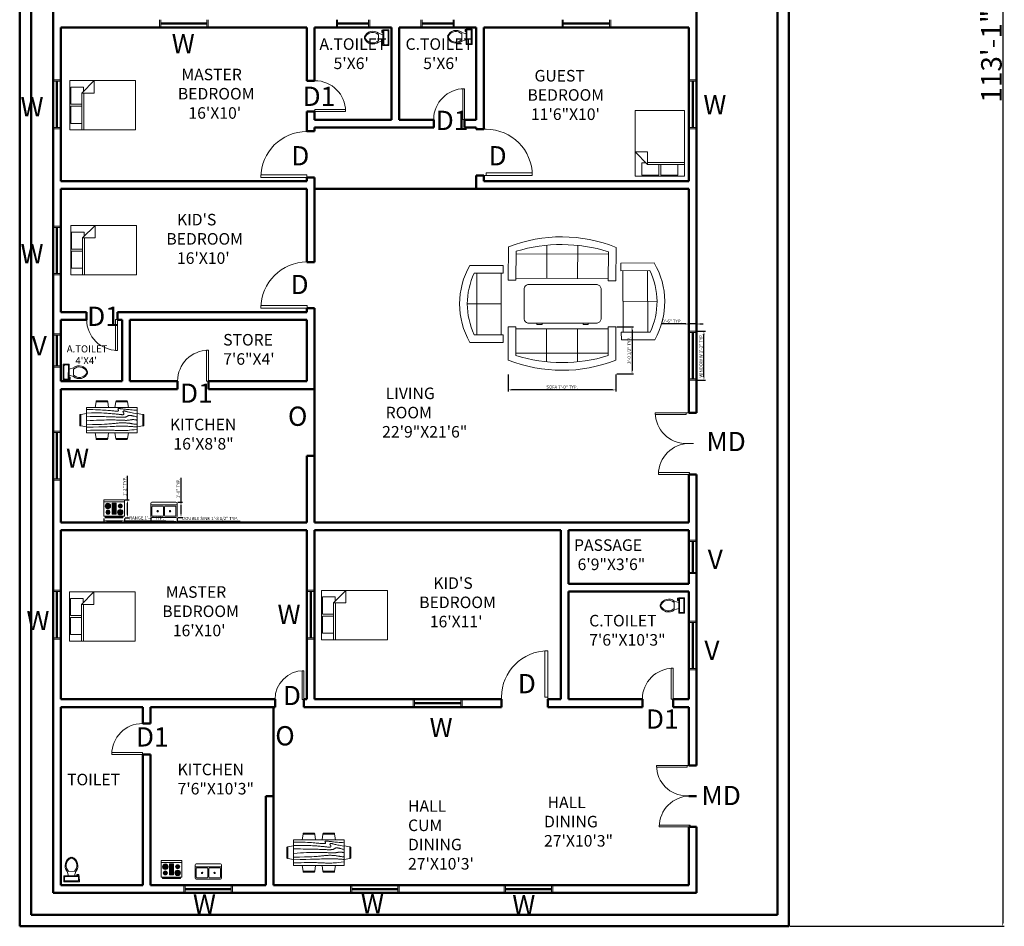
# Model space of a CAD drawing. Units: inches. Extents: x -7040 to -4088, y 6092 to 7645.
# Tile 8 of 11: x -5800 to -5032, y 6157 to 6864. Entities that reach past the tile are written whole.
import ezdxf

# ---------------------------------------------------------------- set-up
doc = ezdxf.new("R2010")
doc.units = ezdxf.units.IN
for name, color, linetype, lineweight in [('A-ANNO-DIMS', 2, 'Continuous', 18), ('A-ANNO-TEXT', 7, 'Continuous', 25), ('A-AREA-IDEN', 3, 'Continuous', 25), ('A-DOOR', 3, 'Continuous', 18), ('A-FLOR-FIXT', 9, 'Continuous', 13), ('A-FURN', 8, 'Continuous', 13), ('A-GLAZ', 4, 'Continuous', 18), ('A-WALL', 7, 'Continuous', 50)]:
    doc.layers.add(name, color=color, linetype=linetype, lineweight=lineweight)
doc.styles.get("Standard").update_dxf_attribs({"font": 'arial.ttf'})
doc.dimstyles.new('ISO-25', dxfattribs={"dimtxt": 2.5, "dimasz": 2.5, "dimexe": 1.25, "dimexo": 0.625, "dimtad": 1, "dimdec": 0, "dimlunit": 3, "dimtxsty": 'Standard', "dimcen": 2.5, "dimadec": 0, "dimazin": 0, "dimtfac": 1, "dimtdec": 0, "dimtmove": 0, "dimatfit": 3, "dimfxl": 1, "dimarcsym": 0})

# ---------------------------------------------------------------- blocks, each defined once
blk = doc.blocks.new('*U8')
for p, q in [((0, 0), (0, -100)), ((750, 0), (750, -100))]:
    blk.add_line(p, q)
blk.add_lwpolyline([(0, 0), (0, 750), (43.75, 750), (43.75, 0)], close=True)
blk.add_arc((0, 0), 750, 0, 90)
blk = doc.blocks.new('Bed - Queen')
for p, q in [((0, -80.00003), (0, 0)), ((0, 0), (59.99999, 0)), ((59.99999, 0), (59.99999, -80.00003)), ((7.99999, -1.2), (28.79998, -1.2)), ((7.99999, -14.4), (7.99999, -1.2)), ((28.79998, -1.2), (28.79998, -14.4)), ((31.19999, -1.2), (51.99999, -1.2)), ((31.19999, -14.4), (31.19999, -1.2)), ((51.99999, -1.2), (51.99999, -16.4)), ((0, -14.4), (44.8, -14.4)), ((44.8, -16.8), (0, -16.8)), ((59.99999, -29.6), (44.8, -14.4)), ((44.8, -14.4), (44.8, -29.6)), ((51.99999, -16.4), (46.79936, -16.4)), ((44.8, -29.6), (59.99999, -29.6)), ((59.99999, -80.00003), (0, -80.00003))]:
    blk.add_line(p, q)
blk = doc.blocks.new('Range-Oven - 30 in top')
for p, q in [((0, -3), (30, -3)), ((12, -6), (18, -6)), ((13, -20), (13, -6)), ((14, -6), (14, -20)), ((15, -20), (15, -6)), ((16, -6), (16, -20)), ((17, -20), (17, -6)), ((6, -24), (6, -25)), ((8, -25), (8, -24)), ((18, -20), (12, -20)), ((22, -25), (22, -24)), ((24, -24), (24, -25))]:
    blk.add_line(p, q)
for points in [[(0, -24), (0, 0), (30, 0), (30, -24)], [(12, -21), (12, -5), (18, -5), (18, -21)], [(2, -26), (2, -25), (28, -25), (28, -26)]]:
    blk.add_lwpolyline(points, close=True)
for centre, radius in [((6, -9), 4), ((6, -9), 3), ((6, -9), 2), ((6, -9), 1), ((24, -18), 4), ((24, -9), 3), ((24, -9), 2), ((24, -9), 1), ((6, -18), 3), ((6, -18), 2), ((6, -18), 1), ((24, -18), 3), ((24, -18), 2), ((24, -18), 1)]:
    blk.add_circle(centre, radius)
blk = doc.blocks.new('Sink-double - 36 in top')
for p, q in [((-18, -4), (18, -4)), ((-0.75, -18.5), (-0.75, -6.5)), ((0.75, -6.5), (0.75, -18.5))]:
    blk.add_line(p, q)
for points in [[(-16.5, 0), (16.5, 0)], [(-18, -19.5), (-18, -1.5)], [(-16.5, -18.5), (-16.5, -6.5)], [(-15.5, -5.5), (-1.75, -5.5)], [(1.75, -5.5), (15.5, -5.5)], [(16.5, -6.5), (16.5, -18.5)], [(18, -1.5), (18, -19.5)], [(16.5, -21), (-16.5, -21)], [(-1.75, -19.5), (-15.5, -19.5)], [(15.5, -19.5), (1.75, -19.5)]]:
    blk.add_lwpolyline(points)
for centre, radius in [((-8.5, -12.5), 1), ((-8.5, -12.5), 0.5), ((8.5, -12.5), 1), ((8.5, -12.5), 0.5)]:
    blk.add_circle(centre, radius)
for centre, radius, start, end in [((-16.5, -1.5), 1.5, 90, 180), ((16.5, -1.5), 1.5, 0, 90), ((-15.5, -6.5), 1, 90, 180), ((-1.75, -6.5), 1, 0, 90), ((1.75, -6.5), 1, 90, 180), ((15.5, -6.5), 1, 0, 90), ((-16.5, -19.5), 1.5, 180, 270), ((-15.5, -18.5), 1, 180, 270), ((-1.75, -18.5), 1, 270, 0), ((1.75, -18.5), 1, 180, 270), ((15.5, -18.5), 1, 270, 0), ((16.5, -19.5), 1.5, 270, 0)]:
    blk.add_arc(centre, radius, start, end)
blk = doc.blocks.new('Toilet - top')
for p, q in [((-10, -8.5), (-8, -8.5)), ((-10, -9.5), (-10, -8.5)), ((-7, -9.5), (-10, -9.5)), ((-8, -8.5), (-8, -8)), ((-7, -8), (-7, -9.5)), ((-4, -8), (-6, -14)), ((4, -8), (6, -14)), ((9.5, -6), (9.5, -2)), ((4, -14), (-4, -14))]:
    blk.add_line(p, q)
blk.add_lwpolyline([(10.5, -8), (10.5, 0), (-10.5, 0), (-10.5, -8)], close=True)
for points in [[(-9.5, -2), (-9.5, -6)], [(8.5, -1), (-8.5, -1)], [(-8.5, -7), (8.5, -7)]]:
    blk.add_lwpolyline(points)
for centre, radius, start, end in [((-8.6, -1.9), 0.884, 81.8699, 188.1301), ((-8.6, -6.1), 0.884, 171.8699, 278.1301), ((8.6, -1.9), 0.884, 351.8699, 98.1301), ((8.6, -6.1), 0.884, 261.8699, 8.1301), ((3.5, -21.6), 12.2, 141.4691, 247.9714), ((4.2, -21.8), 11.3, 136.3677, 238.9468), ((-3.5, -21.6), 12.2, 292.0284, 38.5307), ((-4.2, -21.8), 11.3, 301.053, 43.6321), ((0, -27.9), 4, 245.7318, 294.2682), ((0, -29), 4, 254.8605, 285.1395)]:
    blk.add_arc(centre, radius, start, end)
blk = doc.blocks.new('Dining Set - 36 x 72 in.')
for p, q in [((36, 18), (-36, 18)), ((-36, 18), (-36, -18)), ((-22.2343, 26.00059), (-23.4847, 17.99762)), ((-22.2304, 26), (-5.7608, 26)), ((-22, 27.5), (-22.1562, 26.50042)), ((-5.8416, 26.5), (-22.1534, 26.5)), ((-22, 27.5), (-6, 27.5)), ((-5.8437, 26.49966), (-6, 27.5)), ((-4.5152, 17.99762), (-5.7655, 25.99926)), ((5.7657, 26.00059), (4.5153, 17.99762)), ((5.7696, 26), (22.2392, 26)), ((6, 27.5), (5.8438, 26.50042)), ((22.1584, 26.5), (5.8466, 26.5)), ((6, 27.5), (22, 27.5)), ((22.1563, 26.49966), (22, 27.5)), ((23.4848, 17.99762), (22.2345, 25.99926)), ((36, -18), (36, 18)), ((-45.5, 8), (-44.5004, 8.15617)), ((-45.5, 8), (-45.5, -8)), ((-44.5, -8.15843), (-44.5, 8.15338)), ((-44.0006, 8.23428), (-35.9976, 9.48474)), ((-44, 8.23041), (-44, -8.23915)), ((44.0006, 8.23428), (35.9976, 9.48474)), ((44, 8.23041), (44, -8.23915)), ((44.5, -8.15843), (44.5, 8.15338)), ((45.5, 8), (44.5005, 8.15617)), ((45.5, 8), (45.5, -8)), ((-44.4997, -8.15631), (-45.5, -8)), ((-35.9976, -9.48476), (-43.9993, -8.2345)), ((35.9976, -9.48476), (43.9993, -8.2345)), ((44.4997, -8.15631), (45.5, -8)), ((-36, -18), (36, -18)), ((-22.2343, -26.0006), (-23.4847, -17.99762)), ((-22.2304, -26), (-5.7608, -26)), ((-22, -27.5), (-22.1562, -26.50044)), ((-5.8416, -26.5), (-22.1534, -26.5)), ((-22, -27.5), (-6, -27.5)), ((-5.8437, -26.49967), (-6, -27.5)), ((-4.5152, -17.99762), (-5.7655, -25.99928)), ((5.7657, -26.0006), (4.5153, -17.99762)), ((5.7696, -26), (22.2392, -26)), ((6, -27.5), (5.8438, -26.50044)), ((22.1584, -26.5), (5.8466, -26.5)), ((6, -27.5), (22, -27.5)), ((22.1563, -26.49967), (22, -27.5)), ((23.4848, -17.99762), (22.2345, -25.99928))]:
    blk.add_line(p, q)
for points in [[(-36, 15), (-31.1772, 14.97754), (-26.8079, 14.91406), (-22.8538, 14.81543), (-19.276, 14.6875), (-16.0362, 14.53613), (-13.0957, 14.36718), (-10.4159, 14.18652), (-7.9583, 14), (-5.6904, 13.81315), (-3.6035, 13.63021), (-1.6954, 13.45508), (0.0365, 13.29166), (1.5945, 13.14388), (2.9811, 13.01562), (4.1988, 12.9108), (5.25, 12.83333), (6.1393, 12.78613), (6.8802, 12.76823), (7.4883, 12.77767), (7.9792, 12.8125), (8.3685, 12.87077), (8.6719, 12.95052), (8.9049, 13.0498), (9.0833, 13.16666), (9.2205, 13.29899), (9.3216, 13.44401), (9.3895, 13.59879), (9.4271, 13.76041), (9.4373, 13.92594), (9.4232, 14.09245), (9.3875, 14.257), (9.3333, 14.41666), (9.2638, 14.56917), (9.1836, 14.71484), (9.0975, 14.85465), (9.0104, 14.98958), (8.9272, 15.1206), (8.8529, 15.2487), (8.7922, 15.37483), (8.75, 15.5), (8.7305, 15.62467), (8.7344, 15.74739), (8.7617, 15.86621), (8.8125, 15.97916), (8.8867, 16.08431), (8.9844, 16.17968), (9.1055, 16.26334), (9.25, 16.33333), (9.4189, 16.38802), (9.6172, 16.42708), (9.8506, 16.45052), (10.125, 16.45833), (10.4463, 16.45052), (10.8203, 16.42708), (11.2529, 16.38802), (11.75, 16.33333), (12.3184, 16.26318), (12.9694, 16.17838), (13.7151, 16.07991), (14.5677, 15.96875), (15.5395, 15.84586), (16.6426, 15.71224), (17.8893, 15.56884), (19.2917, 15.41666), (20.859, 15.25667), (22.5879, 15.08984), (24.4721, 14.91715), (26.5052, 14.73958), (28.6809, 14.5581), (30.9929, 14.3737), (33.4347, 14.18733), (36, 14)], [(-36, 10), (-28.9766, 10.14274), (-23.1725, 10.20442), (-18.4241, 10.19775), (-14.5677, 10.13541), (-11.4399, 10.03011), (-8.877, 9.89453), (-6.7154, 9.74137), (-4.7917, 9.58333), (-2.9698, 9.43082), (-1.2246, 9.28515), (0.4415, 9.14534), (2.026, 9.01041), (3.5266, 8.87939), (4.9408, 8.7513), (6.266, 8.62516), (7.5, 8.5), (8.6411, 8.37549), (9.6914, 8.2539), (10.6538, 8.13818), (11.5312, 8.03125), (12.3267, 7.93603), (13.043, 7.85547), (13.6831, 7.79248), (14.25, 7.75), (14.7471, 7.7303), (15.1797, 7.73307), (15.5537, 7.75732), (15.875, 7.80208), (16.1494, 7.86637), (16.3828, 7.94922), (16.5811, 8.04964), (16.75, 8.16666), (16.8944, 8.29915), (17.0143, 8.44531), (17.1089, 8.60319), (17.1771, 8.77083), (17.218, 8.94629), (17.2305, 9.1276), (17.2137, 9.31282), (17.1667, 9.5), (17.0895, 9.6875), (16.987, 9.875), (16.8649, 10.0625), (16.7292, 10.25), (16.5856, 10.4375), (16.4401, 10.625), (16.2985, 10.8125), (16.1667, 11), (16.05, 11.18733), (15.9518, 11.3737), (15.8752, 11.5581), (15.8229, 11.73958), (15.798, 11.91715), (15.8034, 12.08984), (15.842, 12.25667), (15.9167, 12.41666), (16.0295, 12.56836), (16.1784, 12.70833), (16.3605, 12.83268), (16.5729, 12.9375), (16.8127, 13.01888), (17.0768, 13.07291), (17.3625, 13.0957), (17.6667, 13.08333), (17.9894, 13.03312), (18.3418, 12.94726), (18.7382, 12.82918), (19.1927, 12.68229), (19.7195, 12.51001), (20.3327, 12.31575), (21.0465, 12.10294), (21.875, 11.875), (22.8357, 11.63354), (23.959, 11.37304), (25.2786, 11.08618), (26.8282, 10.76562), (28.6414, 10.40405), (30.752, 9.99414), (33.1936, 9.52856), (36, 9)], [(-36, 5.5), (-30.7157, 5.3348), (-26.069, 5.20963), (-21.9946, 5.11767), (-18.4271, 5.05208), (-15.3009, 5.00602), (-12.5508, 4.97265), (-10.1112, 4.94515), (-7.9167, 4.91666), (-5.909, 4.88167), (-4.0586, 4.83984), (-2.3429, 4.79215), (-0.7396, 4.73958), (0.7739, 4.6831), (2.22, 4.6237), (3.6213, 4.56233), (5, 4.5), (6.373, 4.43782), (7.7344, 4.3776), (9.0723, 4.32129), (10.375, 4.27083), (11.6309, 4.22819), (12.8281, 4.19531), (13.9551, 4.17415), (15, 4.16666), (15.954, 4.17448), (16.819, 4.19791), (17.6001, 4.23698), (18.3021, 4.29166), (18.9299, 4.36198), (19.4883, 4.44791), (19.9823, 4.54948), (20.4167, 4.66666), (20.7969, 4.79899), (21.1302, 4.94401), (21.4245, 5.09879), (21.6875, 5.26041), (21.9271, 5.42594), (22.1511, 5.59245), (22.3672, 5.757), (22.5834, 5.91666), (22.8065, 6.06868), (23.0404, 6.21093), (23.2879, 6.34147), (23.5521, 6.45833), (23.8358, 6.55957), (24.142, 6.64323), (24.4735, 6.70735), (24.8334, 6.75), (25.2235, 6.76969), (25.642, 6.76692), (26.0858, 6.74267), (26.5521, 6.69791), (27.0379, 6.63362), (27.5404, 6.55078), (28.0565, 6.45036), (28.5834, 6.33333), (29.1242, 6.19987), (29.7071, 6.04687), (30.3661, 5.87044), (31.1354, 5.66666), (32.0493, 5.43164), (33.142, 5.16146), (34.4475, 4.85221), (36, 4.5)], [(-36, -1), (-30.7915, -0.6591), (-26.0195, -0.38216), (-21.6519, -0.16284), (-17.6563, 0.00521), (-14.0005, 0.12833), (-10.6523, 0.21289), (-7.5796, 0.26522), (-4.75, 0.29166), (-2.134, 0.29793), (0.2878, 0.28711), (2.5317, 0.26163), (4.6146, 0.22396), (6.5529, 0.17651), (8.3633, 0.12174), (10.0623, 0.06209), (11.6667, 0), (13.1899, -0.06201), (14.6341, -0.1211), (15.9982, -0.17432), (17.2813, -0.21875), (18.4823, -0.25147), (19.6003, -0.26953), (20.6343, -0.27002), (21.5834, -0.25), (22.4481, -0.20768), (23.2357, -0.14584), (23.9549, -0.06836), (24.6146, 0.02083), (25.2235, 0.11784), (25.7904, 0.21875), (26.3241, 0.31966), (26.8334, 0.41666), (27.3265, 0.50618), (27.8099, 0.58593), (28.2894, 0.65397), (28.7709, 0.70833), (29.2601, 0.74707), (29.763, 0.76823), (30.2855, 0.76985), (30.8334, 0.75), (31.4088, 0.70784), (31.9994, 0.64713), (32.589, 0.57275), (33.1615, 0.48958), (33.7008, 0.4025), (34.1908, 0.3164), (34.6153, 0.23616), (34.9584, 0.16666), (35.2099, 0.11165), (35.3848, 0.07031), (35.504, 0.04069), (35.5886, 0.02083), (35.6594, 0.00879), (35.7377, 0.0026), (35.8442, 0.00032), (36, 0)], [(-36, -6.5), (-27.1843, -6.31267), (-20.084, -6.1263), (-14.469, -5.9419), (-10.1094, -5.76042), (-6.7752, -5.58285), (-4.2363, -5.41016), (-2.2629, -5.24333), (-0.625, -5.08334), (0.8708, -4.93099), (2.2715, -4.78646), (3.5872, -4.64974), (4.8281, -4.52084), (6.0046, -4.39974), (7.127, -4.28646), (8.2053, -4.18099), (9.25, -4.08334), (10.2705, -3.99382), (11.2734, -3.91407), (12.2647, -3.84603), (13.25, -3.79167), (14.2354, -3.75293), (15.2266, -3.73177), (16.2295, -3.73015), (17.25, -3.75), (18.2912, -3.79248), (19.3451, -3.85547), (20.4009, -3.93604), (21.4479, -4.03125), (22.4754, -4.13819), (23.4727, -4.25391), (24.4289, -4.37549), (25.3334, -4.5), (26.1785, -4.62492), (26.9694, -4.74935), (27.7145, -4.87281), (28.4219, -4.99479), (29.1, -5.11483), (29.7572, -5.23242), (30.4016, -5.34709), (31.0417, -5.45834), (31.6837, -5.56437), (32.3262, -5.65821), (32.9658, -5.73153), (33.599, -5.77604), (34.2224, -5.78345), (34.8327, -5.74545), (35.4264, -5.65373), (36, -5.5)], [(-36, -10), (-26.4022, -9.81299), (-18.4675, -9.62891), (-11.9839, -9.45069), (-6.7396, -9.28125), (-2.5226, -9.12354), (0.8789, -8.98047), (3.6769, -8.85498), (6.0833, -8.75), (8.2767, -8.66765), (10.3021, -8.60677), (12.1712, -8.56543), (13.8958, -8.54167), (15.4876, -8.53353), (16.9583, -8.53907), (18.3197, -8.55632), (19.5834, -8.58334), (20.7616, -8.61841), (21.8685, -8.66081), (22.9188, -8.71004), (23.9271, -8.76563), (24.9081, -8.82707), (25.8763, -8.89388), (26.8465, -8.96558), (27.8334, -9.04167), (28.8474, -9.12118), (29.8828, -9.20117), (30.93, -9.27824), (31.9792, -9.34896), (33.0205, -9.40991), (34.0443, -9.45768), (35.0407, -9.48885), (36, -9.5)], [(-36, -14.5), (-30.0881, -14.33513), (-25.0332, -14.21224), (-20.7312, -14.12647), (-17.0781, -14.07292), (-13.97, -14.04671), (-11.3027, -14.04297), (-8.9724, -14.05681), (-6.875, -14.08334), (-4.9224, -14.11833), (-3.0905, -14.16016), (-1.3709, -14.20785), (0.2448, -14.26042), (1.7647, -14.3169), (3.1973, -14.3763), (4.5507, -14.43767), (5.8333, -14.5), (7.0554, -14.5621), (8.235, -14.62175), (9.3922, -14.67652), (10.5469, -14.72396), (11.7192, -14.76164), (12.929, -14.78711), (14.1965, -14.79794), (15.5417, -14.79167), (16.9933, -14.76424), (18.6152, -14.70508), (20.4804, -14.60197), (22.6615, -14.44271), (25.2312, -14.21509), (28.2624, -13.9069), (31.8277, -13.50594), (36, -13)]]:
    blk.add_lwpolyline(points)
blk = doc.blocks.new('Desk - 30 x 60 in.')
for p, q in [((-26.999995, 0), (26.999995, 0)), ((-29.999995, -27), (-29.999995, -3)), ((29.999995, -3), (29.999995, -27)), ((26.999995, -30), (-26.999995, -30)), ((-20.000005, -30), (-20.000005, -31)), ((-16.000005, -31), (-16.000005, -30)), ((15.999995, -31), (15.999995, -30)), ((19.999995, -30), (19.999995, -31)), ((-20.000005, -31), (-16.000005, -31)), ((19.999995, -31), (15.999995, -31))]:
    blk.add_line(p, q)
for centre, start, end in [((-26.499995, -3.5), 98.1301, 171.8699), ((26.499995, -3.5), 8.130102, 81.8699), ((-26.499995, -26.5), 188.1301, 261.8699), ((26.499995, -26.5), 278.1301, 351.8699)]:
    blk.add_arc(centre, 3.535534, start, end)
blk = doc.blocks.new('Sofa - Roundback 7 ft.')
for p, q in [((-12.00002, -32.4421), (-12.00003, -6.5971)), ((11.99997, -32.4421), (11.99998, -6.5971)), ((-36.000027, -34), (-36.000027, -11.4696)), ((-35.999844, -13.3819), (35.9998, -13.3819)), ((35.99998, -34), (35.99998, -11.4696)), ((-36.000027, -32.4421), (35.99998, -32.4421))]:
    blk.add_line(p, q)
for points in [[(-36.000027, -34), (-42.000027, -34), (-42.000027, -8)], [(41.99998, -8), (41.99998, -34), (35.99998, -34)]]:
    blk.add_lwpolyline(points)
for centre, radius, start, end in [((0, -114.25), 114.25, 68.43141, 111.5686), ((-0.00001, -127.1968), 121.1968, 72.72033, 107.2797)]:
    blk.add_arc(centre, radius, start, end)
blk = doc.blocks.new('Sofa - Roundback Loveseat 5 ft.')
for p, q in [((0, -32.44198), (0, -5.99998)), ((-24, -33.99998), (-24, -11.46958)), ((-23.9998, -13.38178), (23.99986, -13.38178)), ((24.00004, -33.99998), (24.00004, -11.46958)), ((-24, -32.44198), (24.00004, -32.44198))]:
    blk.add_line(p, q)
for points in [[(-24, -33.99998), (-30, -33.99998), (-30, -7.99998)], [(30.00004, -7.99998), (30.00004, -33.99998), (24.00004, -33.99998)]]:
    blk.add_lwpolyline(points)
for centre, radius, start, end in [((0, -60.24998), 60.24998, 60.13715, 119.8628), ((0, -61.38438), 55.38444, 64.32083, 115.6792)]:
    blk.add_arc(centre, radius, start, end)
blk = doc.blocks.new('*D102')
at = {"layer": 'A-ANNO-DIMS', "color": 0, "lineweight": -2, "transparency": 16777216}
for p, q in [((-5199.27, 7513.76), (-5031.95, 7513.76)), ((-5033.2, 7511.26), (-5033.2, 6159.26)), ((-5199.27, 6156.76), (-5031.95, 6156.76))]:
    blk.add_line(p, q, dxfattribs=at)
at = {"layer": 'A-ANNO-DIMS', "color": 0, "transparency": 16777216}
for points in [[(-5033.61, 7511.26), (-5032.78, 7511.26), (-5033.2, 7513.76)], [(-5033.61, 6159.26), (-5032.78, 6159.26), (-5033.2, 6156.76)]]:
    blk.add_solid(points, dxfattribs=at)
at = {"layer": 'Defpoints', "color": 0, "transparency": 16777216}
for p in [(-5199.9, 7513.76), (-5199.9, 6156.76), (-5033.2, 6156.76)]:
    blk.add_point(p, dxfattribs=at)
at = {"layer": 'A-ANNO-DIMS', "color": 0, "transparency": 16777216, "insert": (-5042, 6835.26), "char_height": 2.5, "attachment_point": 5, "rotation": 90}
blk.add_mtext('{\\H6.4x;113\'-1"}', dxfattribs=at)
blk = doc.blocks.new('WIN-36')
for p, q in [((0, 6), (0, 0)), ((1, 6), (1, 0)), ((1, 3.5), (37, 3.5)), ((1, 3), (37, 3)), ((1, 2.5), (37, 2.5)), ((37, 6), (37, 0)), ((38, 6), (38, 0))]:
    blk.add_line(p, q)
blk = doc.blocks.new('WIN-24')
for p, q in [((0, 6), (0, 0)), ((1, 6), (1, 0)), ((1, 3.5), (25, 3.5)), ((1, 3), (25, 3)), ((1, 2.5), (25, 2.5)), ((25, 6), (25, 0)), ((26, 6), (26, 0))]:
    blk.add_line(p, q)
blk = doc.blocks.new('*D114')
at = {"layer": 'A-ANNO-DIMS', "color": 0, "lineweight": -2, "transparency": 16777216}
for p, q in [((-5271.27, 6620.76), (-5264.95, 6620.76)), ((-5266.2, 6585.26), (-5266.2, 6618.26)), ((-5271.27, 6582.76), (-5264.95, 6582.76))]:
    blk.add_line(p, q, dxfattribs=at)
at = {"layer": 'A-ANNO-DIMS', "color": 0, "transparency": 16777216}
for points in [[(-5266.62, 6618.26), (-5265.78, 6618.26), (-5266.2, 6620.76)], [(-5266.62, 6585.26), (-5265.78, 6585.26), (-5266.2, 6582.76)]]:
    blk.add_solid(points, dxfattribs=at)
at = {"layer": 'Defpoints', "color": 0, "transparency": 16777216}
for p in [(-5271.9, 6620.76), (-5266.2, 6620.76), (-5271.9, 6582.76)]:
    blk.add_point(p, dxfattribs=at)
at = {"layer": 'A-ANNO-DIMS', "color": 0, "transparency": 16777216, "insert": (-5268.12, 6601.76), "char_height": 2.5, "attachment_point": 5, "rotation": 90}
blk.add_mtext('WINDOW W 3\'-2" TYP.', dxfattribs=at)
blk = doc.blocks.new('*D115')
at = {"layer": 'A-ANNO-DIMS', "color": 0, "lineweight": -2, "transparency": 16777216}
for p, q in [((-5277.9, 6621.38), (-5277.9, 6627.71)), ((-5271.9, 6621.38), (-5271.9, 6627.71)), ((-5280.4, 6626.46), (-5299.39, 6626.46)), ((-5271.9, 6626.46), (-5277.9, 6626.46)), ((-5269.4, 6626.46), (-5266.9, 6626.46))]:
    blk.add_line(p, q, dxfattribs=at)
at = {"layer": 'A-ANNO-DIMS', "color": 0, "transparency": 16777216}
for points in [[(-5280.4, 6626.88), (-5280.4, 6626.04), (-5277.9, 6626.46)], [(-5269.4, 6626.88), (-5269.4, 6626.04), (-5271.9, 6626.46)]]:
    blk.add_solid(points, dxfattribs=at)
at = {"layer": 'Defpoints', "color": 0, "transparency": 16777216}
for p in [(-5277.9, 6626.46), (-5277.9, 6620.76), (-5271.9, 6620.76)]:
    blk.add_point(p, dxfattribs=at)
at = {"layer": 'A-ANNO-DIMS', "color": 0, "transparency": 16777216, "insert": (-5291.14, 6628.36), "char_height": 2.5, "attachment_point": 5}
blk.add_mtext('0\'-6" TYP.', dxfattribs=at)
blk = doc.blocks.new('*D138')
at = {"layer": 'A-ANNO-DIMS', "color": 0, "lineweight": -2, "transparency": 16777216}
for p, q in [((-5418.91, 6587.05), (-5418.91, 6573.83)), ((-5334.91, 6587.04), (-5334.91, 6573.81)), ((-5337.41, 6575.06), (-5416.41, 6575.08))]:
    blk.add_line(p, q, dxfattribs=at)
at = {"layer": 'A-ANNO-DIMS', "color": 0, "transparency": 16777216}
for points in [[(-5416.41, 6575.49), (-5416.41, 6574.66), (-5418.91, 6575.08)], [(-5337.41, 6575.48), (-5337.41, 6574.64), (-5334.91, 6575.06)]]:
    blk.add_solid(points, dxfattribs=at)
at = {"layer": 'Defpoints', "color": 0, "transparency": 16777216}
for p in [(-5418.91, 6587.68), (-5334.91, 6587.66), (-5418.91, 6575.08)]:
    blk.add_point(p, dxfattribs=at)
at = {"layer": 'A-ANNO-DIMS', "color": 0, "transparency": 16777216, "insert": (-5376.91, 6576.99), "char_height": 2.5, "attachment_point": 5, "rotation": 359.98844}
blk.add_mtext('SOFA 7\'-0" TYP.', dxfattribs=at)
blk = doc.blocks.new('*D139')
at = {"layer": 'A-ANNO-DIMS', "color": 0, "lineweight": -2, "transparency": 16777216}
for p, q in [((-5334.28, 6624.33), (-5321.05, 6624.32)), ((-5322.3, 6621.82), (-5322.31, 6590.16)), ((-5334.28, 6587.66), (-5321.06, 6587.66))]:
    blk.add_line(p, q, dxfattribs=at)
at = {"layer": 'A-ANNO-DIMS', "color": 0, "transparency": 16777216}
for points in [[(-5322.72, 6621.82), (-5321.88, 6621.82), (-5322.3, 6624.32)], [(-5322.72, 6590.16), (-5321.89, 6590.16), (-5322.31, 6587.66)]]:
    blk.add_solid(points, dxfattribs=at)
at = {"layer": 'Defpoints', "color": 0, "transparency": 16777216}
for p in [(-5334.9, 6624.33), (-5334.91, 6587.66), (-5322.31, 6587.66)]:
    blk.add_point(p, dxfattribs=at)
at = {"layer": 'A-ANNO-DIMS', "color": 0, "transparency": 16777216, "insert": (-5324.22, 6605.99), "char_height": 2.5, "attachment_point": 5, "rotation": 89.98844}
blk.add_mtext('3\'-0 1/2" TYP.', dxfattribs=at)
blk = doc.blocks.new('*D150')
at = {"layer": 'A-ANNO-DIMS', "color": 0, "lineweight": -2, "transparency": 16777216}
for p, q in [((-5734.29, 6474.79), (-5734.29, 6471.76)), ((-5718.26, 6474.79), (-5718.26, 6471.76)), ((-5731.79, 6473.01), (-5720.76, 6473.01)), ((-5718.26, 6473.01), (-5686.01, 6473.01))]:
    blk.add_line(p, q, dxfattribs=at)
at = {"layer": 'A-ANNO-DIMS', "color": 0, "transparency": 16777216}
for points in [[(-5731.79, 6473.42), (-5731.79, 6472.59), (-5734.29, 6473.01)], [(-5720.76, 6473.42), (-5720.76, 6472.59), (-5718.26, 6473.01)]]:
    blk.add_solid(points, dxfattribs=at)
at = {"layer": 'Defpoints', "color": 0, "transparency": 16777216}
for p in [(-5734.29, 6475.41), (-5718.26, 6475.41), (-5718.26, 6473.01)]:
    blk.add_point(p, dxfattribs=at)
at = {"layer": 'A-ANNO-DIMS', "color": 0, "transparency": 16777216, "insert": (-5700.89, 6474.92), "char_height": 2.5, "attachment_point": 5}
blk.add_mtext('RANGE 1\'-4" TYP.', dxfattribs=at)
blk = doc.blocks.new('*D151')
at = {"layer": 'A-ANNO-DIMS', "color": 0, "lineweight": -2, "transparency": 16777216}
for p, q in [((-5715.86, 6489.31), (-5715.86, 6508.06)), ((-5717.64, 6489.31), (-5714.61, 6489.31)), ((-5715.86, 6477.91), (-5715.86, 6486.81)), ((-5717.64, 6475.41), (-5714.61, 6475.41))]:
    blk.add_line(p, q, dxfattribs=at)
at = {"layer": 'A-ANNO-DIMS', "color": 0, "transparency": 16777216}
for points in [[(-5716.27, 6486.81), (-5715.44, 6486.81), (-5715.86, 6489.31)], [(-5716.27, 6477.91), (-5715.44, 6477.91), (-5715.86, 6475.41)]]:
    blk.add_solid(points, dxfattribs=at)
at = {"layer": 'Defpoints', "color": 0, "transparency": 16777216}
for p in [(-5718.26, 6489.31), (-5715.86, 6489.31), (-5718.26, 6475.41)]:
    blk.add_point(p, dxfattribs=at)
at = {"layer": 'A-ANNO-DIMS', "color": 0, "transparency": 16777216, "insert": (-5717.74, 6499.93), "char_height": 2.5, "attachment_point": 5, "rotation": 90}
blk.add_mtext('1\'-2" TYP.', dxfattribs=at)
blk = doc.blocks.new('*D156')
at = {"layer": 'A-ANNO-DIMS', "color": 0, "lineweight": -2, "transparency": 16777216}
for p, q in [((-5697.65, 6475.03), (-5697.65, 6471.33)), ((-5677.16, 6475.03), (-5677.16, 6471.33)), ((-5695.15, 6472.58), (-5679.66, 6472.58)), ((-5677.16, 6472.58), (-5628.01, 6472.58))]:
    blk.add_line(p, q, dxfattribs=at)
at = {"layer": 'A-ANNO-DIMS', "color": 0, "transparency": 16777216}
for points in [[(-5695.15, 6472.99), (-5695.15, 6472.16), (-5697.65, 6472.58)], [(-5679.66, 6472.99), (-5679.66, 6472.16), (-5677.16, 6472.58)]]:
    blk.add_solid(points, dxfattribs=at)
at = {"layer": 'Defpoints', "color": 0, "transparency": 16777216}
for p in [(-5697.65, 6475.65), (-5677.16, 6475.65), (-5677.16, 6472.58)]:
    blk.add_point(p, dxfattribs=at)
at = {"layer": 'A-ANNO-DIMS', "color": 0, "transparency": 16777216, "insert": (-5651.34, 6474.5), "char_height": 2.5, "attachment_point": 5}
blk.add_mtext('DOUBLE SINK 1\'-8 1/2" TYP.', dxfattribs=at)
blk = doc.blocks.new('*D157')
at = {"layer": 'A-ANNO-DIMS', "color": 0, "lineweight": -2, "transparency": 16777216}
for p, q in [((-5674.08, 6487.6), (-5674.08, 6506.36)), ((-5676.53, 6487.6), (-5672.83, 6487.6)), ((-5674.08, 6478.15), (-5674.08, 6485.1)), ((-5676.53, 6475.65), (-5672.83, 6475.65))]:
    blk.add_line(p, q, dxfattribs=at)
at = {"layer": 'A-ANNO-DIMS', "color": 0, "transparency": 16777216}
for points in [[(-5674.5, 6485.1), (-5673.67, 6485.1), (-5674.08, 6487.6)], [(-5674.5, 6478.15), (-5673.67, 6478.15), (-5674.08, 6475.65)]]:
    blk.add_solid(points, dxfattribs=at)
at = {"layer": 'Defpoints', "color": 0, "transparency": 16777216}
for p in [(-5677.16, 6487.6), (-5674.08, 6487.6), (-5677.16, 6475.65)]:
    blk.add_point(p, dxfattribs=at)
at = {"layer": 'A-ANNO-DIMS', "color": 0, "transparency": 16777216, "insert": (-5675.99, 6498.23), "char_height": 2.5, "attachment_point": 5, "rotation": 90}
blk.add_mtext('1\'-0" TYP.', dxfattribs=at)

msp = doc.modelspace()

# ---------------------------------------------------------------- linework, layer by layer
at = {"layer": 'A-WALL'}
for p, q in [((-5799.9, 6156.76), (-5799.9, 7513.76)), ((-5199.9, 7513.76), (-5199.9, 6156.76)), ((-5790.9, 6165.76), (-5790.9, 7504.76)), ((-5208.9, 7504.76), (-5208.9, 6165.76)), ((-5773.9, 6182.76), (-5773.9, 7487.76)), ((-5271.9, 7013.76), (-5271.9, 6557.18)), ((-5767.9, 6857.76), (-5575.9, 6857.76)), ((-5767.9, 6737.76), (-5767.9, 6857.76)), ((-5575.9, 6816.21), (-5575.9, 6857.76)), ((-5575.9, 6816.21), (-5575.9, 6857.76)), ((-5569.9, 6857.76), (-5509.9, 6857.76)), ((-5569.9, 6816.21), (-5569.9, 6857.76)), ((-5569.9, 6816.21), (-5569.9, 6857.76)), ((-5509.9, 6785.76), (-5509.9, 6857.76)), ((-5503.9, 6785.76), (-5503.9, 6857.76)), ((-5503.9, 6857.76), (-5443.9, 6857.76)), ((-5443.9, 6785.76), (-5443.9, 6857.76)), ((-5437.9, 6857.76), (-5277.9, 6857.76)), ((-5437.9, 6778.28), (-5437.9, 6857.76)), ((-5277.9, 6857.76), (-5277.9, 6737.76)), ((-5575.9, 6816.21), (-5569.9, 6816.21)), ((-5575.9, 6792.21), (-5569.9, 6792.21)), ((-5575.9, 6776.8), (-5575.9, 6792.21)), ((-5575.9, 6776.8), (-5575.9, 6792.21)), ((-5569.9, 6785.76), (-5569.9, 6792.21)), ((-5569.9, 6785.76), (-5569.9, 6792.21)), ((-5569.9, 6785.76), (-5509.9, 6785.76)), ((-5503.9, 6785.76), (-5476.99, 6785.76)), ((-5476.99, 6785.76), (-5476.99, 6779.76)), ((-5452.99, 6785.76), (-5452.99, 6779.76)), ((-5452.99, 6785.76), (-5443.9, 6785.76)), ((-5575.9, 6776.8), (-5569.9, 6776.8)), ((-5569.9, 6779.76), (-5509.9, 6779.76)), ((-5569.9, 6776.8), (-5569.9, 6779.76)), ((-5569.9, 6776.8), (-5569.9, 6779.76)), ((-5509.9, 6779.76), (-5476.99, 6779.76)), ((-5452.99, 6779.76), (-5443.9, 6779.76)), ((-5443.9, 6778.28), (-5443.9, 6779.76)), ((-5443.9, 6778.28), (-5437.9, 6778.28)), ((-5767.9, 6737.76), (-5575.9, 6737.76)), ((-5575.9, 6737.76), (-5575.9, 6740.8)), ((-5575.9, 6737.76), (-5575.9, 6740.8)), ((-5575.9, 6740.8), (-5569.9, 6740.8)), ((-5569.9, 6731.76), (-5569.9, 6740.8)), ((-5569.9, 6674.74), (-5569.9, 6740.8)), ((-5443.9, 6731.76), (-5443.9, 6742.28)), ((-5443.9, 6742.28), (-5437.9, 6742.28)), ((-5437.9, 6737.76), (-5437.9, 6742.28)), ((-5437.9, 6737.76), (-5277.9, 6737.76)), ((-5767.9, 6731.76), (-5575.9, 6731.76)), ((-5767.9, 6635.76), (-5767.9, 6731.76)), ((-5575.9, 6674.74), (-5575.9, 6731.76)), ((-5569.9, 6731.76), (-5277.9, 6731.76)), ((-5277.9, 6731.76), (-5277.9, 6557.18)), ((-5575.9, 6674.74), (-5569.9, 6674.74)), ((-5767.9, 6635.76), (-5747.72, 6635.76)), ((-5747.72, 6629.76), (-5747.72, 6635.76)), ((-5723.72, 6629.76), (-5723.72, 6635.76)), ((-5723.72, 6635.76), (-5575.9, 6635.76)), ((-5575.9, 6635.76), (-5575.9, 6638.74)), ((-5575.9, 6638.74), (-5569.9, 6638.74)), ((-5569.9, 6575.76), (-5569.9, 6638.74)), ((-5767.9, 6629.76), (-5747.72, 6629.76)), ((-5767.9, 6581.76), (-5767.9, 6629.76)), ((-5723.72, 6629.76), (-5719.9, 6629.76)), ((-5719.9, 6581.76), (-5719.9, 6629.76)), ((-5713.9, 6581.76), (-5713.9, 6629.76)), ((-5713.9, 6629.76), (-5575.9, 6629.76)), ((-5575.9, 6581.76), (-5575.9, 6629.76)), ((-5767.9, 6581.76), (-5719.9, 6581.76)), ((-5713.9, 6581.76), (-5676.74, 6581.76)), ((-5676.74, 6581.76), (-5676.74, 6575.76)), ((-5652.74, 6581.76), (-5652.74, 6575.76)), ((-5652.74, 6581.76), (-5575.9, 6581.76)), ((-5767.9, 6575.76), (-5676.74, 6575.76)), ((-5767.9, 6471.76), (-5767.9, 6575.76)), ((-5652.74, 6575.76), (-5569.9, 6575.76)), ((-5569.9, 6523.76), (-5569.9, 6575.76)), ((-5277.9, 6557.18), (-5271.9, 6557.18)), ((-5575.9, 6471.76), (-5575.9, 6523.76)), ((-5575.9, 6523.76), (-5569.9, 6523.76)), ((-5569.9, 6471.76), (-5569.9, 6523.76)), ((-5277.9, 6509.18), (-5271.9, 6509.18)), ((-5277.9, 6509.18), (-5277.9, 6471.76)), ((-5271.9, 6509.18), (-5271.9, 6282.26)), ((-5767.9, 6471.76), (-5575.9, 6471.76)), ((-5569.9, 6471.76), (-5277.9, 6471.76)), ((-5767.9, 6465.76), (-5575.9, 6465.76)), ((-5767.9, 6333.76), (-5767.9, 6465.76)), ((-5575.9, 6333.76), (-5575.9, 6465.76)), ((-5569.9, 6333.76), (-5569.9, 6465.76)), ((-5569.9, 6465.76), (-5377.9, 6465.76)), ((-5377.9, 6333.76), (-5377.9, 6465.76)), ((-5371.9, 6423.76), (-5371.9, 6465.76)), ((-5371.9, 6465.76), (-5277.9, 6465.76)), ((-5277.9, 6465.76), (-5277.9, 6423.76)), ((-5371.9, 6423.76), (-5277.9, 6423.76)), ((-5371.9, 6333.76), (-5371.9, 6417.76)), ((-5371.9, 6417.76), (-5277.9, 6417.76)), ((-5277.9, 6417.76), (-5277.9, 6333.76)), ((-5767.9, 6333.76), (-5600.74, 6333.76)), ((-5600.74, 6333.76), (-5600.74, 6327.76)), ((-5578.4, 6333.76), (-5578.4, 6327.76)), ((-5578.4, 6333.76), (-5575.9, 6333.76)), ((-5569.9, 6333.76), (-5424.09, 6333.76)), ((-5424.09, 6333.76), (-5424.09, 6327.76)), ((-5388.09, 6333.76), (-5388.09, 6327.76)), ((-5388.09, 6333.76), (-5377.9, 6333.76)), ((-5371.9, 6333.76), (-5314.26, 6333.76)), ((-5314.26, 6333.76), (-5314.26, 6327.76)), ((-5290.26, 6333.76), (-5290.26, 6327.76)), ((-5290.26, 6333.76), (-5277.9, 6333.76)), ((-5767.9, 6188.76), (-5767.9, 6327.76)), ((-5767.9, 6327.76), (-5703.9, 6327.76)), ((-5703.9, 6327.76), (-5703.9, 6314.86)), ((-5697.9, 6327.76), (-5697.9, 6314.86)), ((-5697.9, 6327.76), (-5601.9, 6327.76)), ((-5601.9, 6327.76), (-5600.74, 6327.76)), ((-5601.9, 6258.26), (-5601.9, 6327.76)), ((-5578.4, 6327.76), (-5424.09, 6327.76)), ((-5388.09, 6327.76), (-5314.26, 6327.76)), ((-5290.26, 6327.76), (-5277.9, 6327.76)), ((-5277.9, 6327.76), (-5277.9, 6282.26)), ((-5703.9, 6314.86), (-5697.9, 6314.86)), ((-5703.9, 6290.86), (-5697.9, 6290.86)), ((-5703.9, 6290.86), (-5703.9, 6188.76)), ((-5697.9, 6290.86), (-5697.9, 6188.76)), ((-5277.9, 6282.26), (-5271.9, 6282.26)), ((-5607.9, 6258.26), (-5607.9, 6188.76)), ((-5607.9, 6258.26), (-5601.9, 6258.26)), ((-5601.9, 6258.26), (-5601.9, 6188.76)), ((-5277.9, 6258.26), (-5271.9, 6258.26)), ((-5277.9, 6234.26), (-5271.9, 6234.26)), ((-5277.9, 6234.26), (-5277.9, 6188.76)), ((-5271.9, 6234.26), (-5271.9, 6182.76)), ((-5271.9, 6182.76), (-5773.9, 6182.76)), ((-5703.9, 6188.76), (-5767.9, 6188.76)), ((-5607.9, 6188.76), (-5697.9, 6188.76)), ((-5277.9, 6188.76), (-5601.9, 6188.76)), ((-5773.9, 6165.76), (-5790.9, 6165.76)), ((-5271.9, 6165.76), (-5773.9, 6165.76)), ((-5208.9, 6165.76), (-5271.9, 6165.76)), ((-5199.9, 6156.76), (-5799.9, 6156.76))]:
    msp.add_line(p, q, dxfattribs=at)

# ---------------------------------------------------------------- block references
at = {"layer": 'A-DOOR'}
for p, xscale, yscale, zscale, rotation in [((-5569.7, 6792.21), -0.0320000014720848, 0.0320000014720848, 0.0320000014720848, 270), ((-5575.85, 6740.6), 0.0479999999999998, 0.0479999999999998, 0.0479999999999998, 90), ((-5436.1, 6742.28), -0.0480000008832502, 0.0480000008832502, 0.0480000008832502, 270), ((-5575.78, 6638.83), 0.0479999999999998, 0.0479999999999998, 0.0479999999999998, 90), ((-5723.69, 6629.84), 0.0319325753922831, 0.0319325753922831, 0.0319325753922831, 180), ((-5280.06, 6557.28), -0.032106775189528, 0.032106775189528, 0.032106775189528, 90), ((-5277.59, 6509.2), 0.0321136266787739, 0.0321136266787739, 0.0321136266787739, 90.00000000000003), ((-5704.13, 6290.86), 0.0319999999999999, 0.0319999999999999, 0.0319999999999999, 90), ((-5279.43, 6282.17), -0.0316755286300598, 0.0316755286300598, 0.0316755286300598, 90), ((-5276.99, 6234.26), 0.0321136266787739, 0.0321136266787739, 0.0321136266787739, 90.00000000000003)]:
    msp.add_blockref('*U8', p, dxfattribs=dict(at, xscale=xscale, yscale=yscale, zscale=zscale, rotation=rotation))
for p, xscale, yscale, zscale in [((-5452.99, 6785.96), -0.0319999999999999, 0.0319999999999999, 0.0319999999999999), ((-5652.74, 6581.96), -0.032, 0.032, 0.032), ((-5388.09, 6335.56), -0.0479999947493871, 0.0479999947493871, 0.0479999947493871), ((-5578.4, 6333.74), -0.0297825006720037, 0.0297825006720037, 0.0297825006720037), ((-5290.26, 6333.96), -0.0319999967421584, 0.0319999967421584, 0.0319999967421584)]:
    msp.add_blockref('*U8', p, dxfattribs=dict(at, xscale=xscale, yscale=yscale, zscale=zscale))
at = {"layer": 'A-FLOR-FIXT', "xscale": 0.5781895628236116, "yscale": 0.5781895628236116, "zscale": 0.5781895628236116}
for p, rotation in [((-5511.96, 6849.76), 270.0514378338742), ((-5447.08, 6850.42), 270.0514378338742), ((-5765.97, 6589.01), 89.40198668992271), ((-5281.28, 6406.91), 270.0514378338742), ((-5759.44, 6191.54), 180.2292282917401)]:
    msp.add_blockref('Toilet - top', p, dxfattribs=dict(at, rotation=rotation))
at = {"layer": 'A-FLOR-FIXT'}
for name, p, xscale, yscale, zscale in [('Range-Oven - 30 in top', (-5734.29, 6489.31), 0.5343739847293781, 0.5343739847293781, 0.5343739847293781), ('Sink-double - 36 in top', (-5687.4, 6487.6), 0.5691595575351838, 0.5691595575351838, 0.5691595575351838), ('Range-Oven - 30 in top', (-5689.53, 6208.02), 0.5343739847293781, 0.5343739847293781, 0.5343739847293781), ('Sink-double - 36 in top', (-5652.77, 6205.53), 0.5691595575351838, 0.5691595575351838, 0.5691595575351838)]:
    msp.add_blockref(name, p, dxfattribs=dict(at, xscale=xscale, yscale=yscale, zscale=zscale))
at = {"layer": 'A-FURN', "xscale": 0.6408536689007259, "yscale": 0.6408536689007259, "zscale": 0.6408536689007259}
for p, rotation in [((-5760.75, 6777.79), 90), ((-5281.43, 6741.62), 180), ((-5760.13, 6664.86), 90), ((-5761.02, 6379.06), 90), ((-5564.38, 6380.27), 90)]:
    msp.add_blockref('Bed - Queen', p, dxfattribs=dict(at, rotation=rotation))
at = {"layer": 'A-FURN'}
for name, p, rotation in [('Sofa - Roundback 7 ft.', (-5376.64, 6694.42), 359.7066467141563), ('Sofa - Roundback Loveseat 5 ft.', (-5296.82, 6644.2), 270.3571450594314), ('Sofa - Roundback Loveseat 5 ft.', (-5456.8, 6642.13), 90.00814269742376), ('Sofa - Roundback 7 ft.', (-5376.91, 6590.34), 179.9884368603272)]:
    msp.add_blockref(name, p, dxfattribs=dict(at, rotation=rotation))
msp.add_blockref('Desk - 30 x 60 in.', (-5376.46, 6657.17), dxfattribs=at)
at = {"layer": 'A-FURN', "xscale": 0.5507153893551977, "yscale": 0.5507153893551977, "zscale": 0.5507153893551977}
for p in [(-5728.06, 6551.47), (-5566.59, 6214.19)]:
    msp.add_blockref('Dining Set - 36 x 72 in.', p, dxfattribs=at)
at = {"layer": 'A-GLAZ'}
for p in [(-5690.9, 6857.76), (-5376.9, 6857.76), (-5492.9, 6327.76), (-5671.9, 6182.76), (-5541.9, 6182.76), (-5422.07, 6182.76)]:
    msp.add_blockref('WIN-36', p, dxfattribs=at)
for name, p, rotation in [('WIN-24', (-5526.9, 6863.76), 180), ('WIN-24', (-5460.9, 6863.76), 180), ('WIN-36', (-5767.9, 6778.76), 90.00000000000082), ('WIN-36', (-5271.9, 6778.76), 90.00000000000082), ('WIN-36', (-5767.9, 6664.76), 89.99999999999817), ('WIN-36', (-5271.9, 6582.76), 90.00000000000044), ('WIN-24', (-5773.9, 6618.76), 269.9999999999953), ('WIN-36', (-5767.9, 6504.76), 89.99999999999817), ('WIN-24', (-5277.9, 6457.76), 269.9999999999924), ('WIN-36', (-5767.9, 6380.76), 89.99999999999775), ('WIN-36', (-5569.9, 6380.76), 89.9999999999955), ('WIN-36', (-5271.9, 6356.76), 90.00000000000044)]:
    msp.add_blockref(name, p, dxfattribs=dict(at, rotation=rotation))

# ---------------------------------------------------------------- texts
at = {"layer": 'A-ANNO-TEXT', "char_height": 15, "attachment_point": 1}
for s, insert in [('{W}', (-5681.35, 6852.62)), ('{D1}', (-5579.24, 6811.52)), ('{W}', (-5266.69, 6805.06)), ('{W}', (-5799.25, 6803.37)), ('{D1}', (-5475.41, 6792.73)), ('{D}', (-5588.08, 6765.14)), ('{D}', (-5434.18, 6765.14)), ('{W}', (-5799.25, 6688.82)), ('{D}', (-5588.63, 6664.76)), ('{D1}', (-5747.26, 6639.94)), ('{V}', (-5790.53, 6617.05)), ('{D1}', (-5674.85, 6580.01)), ('{O}', (-5590.67, 6562.02)), ('{MD}', (-5264.27, 6542.3)), ('{W}', (-5763.74, 6529.33)), ('{V}', (-5263.26, 6450.51)), ('{W}', (-5598.82, 6407.51)), ('{W}', (-5794.65, 6402.75)), ('{V}', (-5265.88, 6379.48)), ('{D}', (-5411.4, 6353.49)), ('{D}', (-5594.64, 6344.22)), ('{D1}', (-5311.46, 6325.87)), ('{O}', (-5600.56, 6312.84)), ('{W}', (-5480.21, 6319.29)), ('{D1}', (-5709.24, 6311.96)), ('{MD}', (-5268.12, 6266.26)), ('{W}', (-5664.8, 6181.74)), ('{W}', (-5533.76, 6181.87)), ('{W}', (-5415.71, 6181.07))]:
    msp.add_mtext_dynamic_manual_height_columns(s, width=1030.7133, gutter_width=12.5, heights=[0], dxfattribs=dict(at, insert=insert))
at = {"layer": 'A-AREA-IDEN', "attachment_point": 1}
for s, insert, char_height in [("{   A.TOILET\\P       5'X6'}", (-5574.34, 6849.25), 9), ("{ C.TOILET\\P      5'X6'}", (-5501.68, 6849.25), 9), ("{ MASTER\\PBEDROOM\\P   16'X10'}", (-5676.53, 6825.53), 9), ('{  GUEST\\PBEDROOM\\P 11\'6"X10\'}', (-5403.86, 6824.56), 9), ("{   KID'S\\PBEDROOM\\P   16'X10'}", (-5685.48, 6712.35), 9), ('{STORE\\P7\'6"X4\'}', (-5641.18, 6618.66), 9), ("{ A.TOILET\\P     4'X4'}", (-5764.85, 6609.76), 5.4718), ('{ LIVING\\P ROOM^J22\'9"X21\'6"}', (-5517.19, 6576.89), 9), ('{KITCHEN\\P 16\'X8\'8"}', (-5682.73, 6552.56), 9), ('{ PASSAGE\\P  6\'9"X3\'6"}', (-5370.27, 6458.54), 9), ("{    KID'S\\PBEDROOM\\P   16'X11'}", (-5488.27, 6428.9), 9), ("{ MASTER\\PBEDROOM\\P   16'X10'}", (-5688.71, 6421.94), 9), ('{ C.TOILET\\P 7\'6"X10\'3"}', (-5358.47, 6399.62), 9), ('{KITCHEN\\P7\'6"X10\'3"}', (-5676.76, 6283.58), 9), ('{TOILET}', (-5762.92, 6275.71), 9), ("{ HALL^J CUM\\P DINING\\P 27'X10'3'}", (-5499.74, 6255.03), 9), ('{ HALL\\PDINING\\P27\'X10\'3"}', (-5390.9, 6257.92), 9)]:
    msp.add_mtext_dynamic_manual_height_columns(s, width=1231.1944, gutter_width=12.5, heights=[0], dxfattribs=dict(at, insert=insert, char_height=char_height))

# ---------------------------------------------------------------- dimensions: what is measured, and where the dimension line sits
at = {"layer": 'A-ANNO-DIMS'}
for base, p1, p2, angle, text, override, picture, middle in [((-5033.2, 6156.76), (-5199.9, 7513.76), (-5199.9, 6156.76), 90, '{\\H6.4x;<>}', {"dimclrd": 0, "dimclre": 0, "dimclrt": 0}, '*D102', (-5042, 6835.26)), ((-5277.9, 6626.46), (-5271.9, 6620.76), (-5277.9, 6620.76), 180, '<> TYP.', {"dimdec": 1, "dimrnd": 0, "dimzin": 1, "dimlunit": 4, "dimfrac": 2}, '*D115', (-5291.14, 6628.36)), ((-5322.31, 6587.66), (-5334.9, 6624.33), (-5334.91, 6587.66), 269.98844, '<> TYP.', {"dimdec": 1, "dimrnd": 0, "dimzin": 1, "dimlunit": 4, "dimfrac": 2}, '*D139', (-5324.22, 6605.99)), ((-5266.2, 6620.76), (-5271.9, 6582.76), (-5271.9, 6620.76), 90, 'WINDOW W <> TYP.', {"dimdec": 1, "dimrnd": 0, "dimzin": 1, "dimlunit": 4, "dimfrac": 2}, '*D114', (-5268.12, 6601.76)), ((-5418.91, 6575.08), (-5334.91, 6587.66), (-5418.91, 6587.68), 179.98844, 'SOFA <> TYP.', {"dimdec": 1, "dimrnd": 0, "dimzin": 1, "dimlunit": 4, "dimfrac": 2}, '*D138', (-5376.91, 6576.99)), ((-5715.86, 6489.31), (-5718.26, 6475.41), (-5718.26, 6489.31), 90, '<> TYP.', {"dimdec": 1, "dimrnd": 0, "dimzin": 1, "dimlunit": 4, "dimfrac": 2}, '*D151', (-5717.74, 6499.93)), ((-5674.0839, 6487.6033), (-5677.1573, 6475.6509), (-5677.1573, 6487.6033), 90, '<> TYP.', {"dimdec": 1, "dimrnd": 0, "dimzin": 1, "dimlunit": 4, "dimfrac": 2}, '*D157', (-5675.9853, 6498.23))]:
    dim = msp.add_linear_dim(base=base, p1=p1, p2=p2, angle=angle, text=text, dimstyle='ISO-25', override=override, dxfattribs=at)
    dim.commit()
    dim.dimension.update_dxf_attribs({"geometry": picture, "text_midpoint": middle})
for base, p1, p2, text, picture, middle in [((-5677.16, 6472.58), (-5697.65, 6475.65), (-5677.16, 6475.65), 'DOUBLE SINK <> TYP.', '*D156', (-5651.34, 6474.5)), ((-5718.26, 6473.01), (-5734.29, 6475.41), (-5718.26, 6475.41), 'RANGE <> TYP.', '*D150', (-5700.89, 6474.92))]:
    dim = msp.add_linear_dim(base=base, p1=p1, p2=p2, text=text, dimstyle='ISO-25', override={"dimdec": 1, "dimrnd": 0, "dimzin": 1, "dimlunit": 4, "dimfrac": 2}, dxfattribs=at)
    dim.commit()
    dim.dimension.update_dxf_attribs({"geometry": picture, "text_midpoint": middle})

doc.saveas('drawing.dxf')
